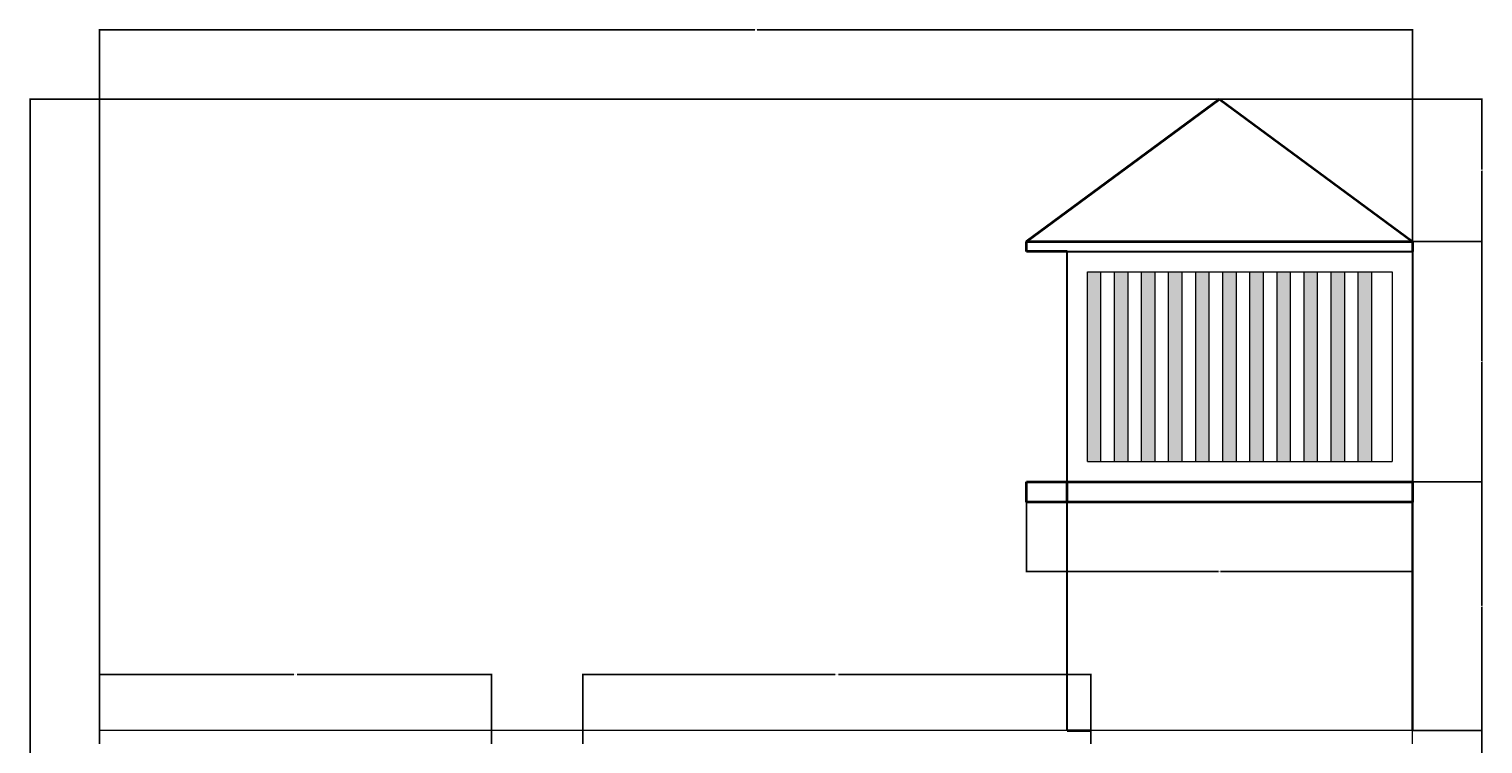
# Model space of a CAD drawing. Units: inches. Extents: x 2156 to 3149, y 1513 to 2286.
# Tile 5 of 5: x 2720 to 3149, y 2075 to 2286. Entities that reach past the tile are written whole.
import ezdxf

# ---------------------------------------------------------------- set-up
doc = ezdxf.new("R2010")
doc.units = ezdxf.units.IN
for name, color, linetype, lineweight in [('A-ANNO-DIMS', 2, 'Continuous', 18), ('A-ELEV', 7, 'Continuous', 30), ('A-ELEV-GLAZ', 4, 'Continuous', 18), ('A-ELEV-GLAZ-PATT', 18, 'Continuous', 13), ('A-ELEV-TRIM', 7, 'Continuous', 20), ('A-ROOF', 7, 'Continuous', 35)]:
    doc.layers.add(name, color=color, linetype=linetype, lineweight=lineweight)
doc.styles.get("Standard").update_dxf_attribs({"font": 'arial.ttf'})
doc.dimstyles.get("Standard").update_dxf_attribs({"dimtxt": 0.18, "dimasz": 0.18, "dimexe": 0.18, "dimexo": 0.0625, "dimgap": 0.09, "dimtad": 0, "dimtih": 1, "dimtoh": 1, "dimdec": 4, "dimzin": 0, "dimdsep": 46, "dimtxsty": 'Standard', "dimcen": 0.09, "dimadec": 0, "dimazin": 0, "dimtfac": 1, "dimtdec": 4, "dimtofl": 0, "dimtmove": 0, "dimatfit": 3, "dimfxl": 1, "dimtolj": 1, "dimtzin": 0, "dimarcsym": 0})

# ---------------------------------------------------------------- blocks, each defined once
blk = doc.blocks.new('*D45')
at = {"layer": 'A-ANNO-DIMS', "color": 0, "lineweight": -2, "transparency": 16777216}
for p, q in [((2740.82, 2078.77), (2740.82, 2285.77)), ((2741, 2285.59), (2934.28, 2285.59)), ((3128.35, 2285.59), (2935.06, 2285.59)), ((3128.53, 2223.16), (3128.53, 2285.77))]:
    blk.add_line(p, q, dxfattribs=at)
at = {"layer": 'A-ANNO-DIMS', "color": 0, "transparency": 16777216}
for points in [[(2741, 2285.62), (2741, 2285.56), (2740.82, 2285.59)], [(3128.35, 2285.62), (3128.35, 2285.56), (3128.53, 2285.59)]]:
    blk.add_solid(points, dxfattribs=at)
at = {"layer": 'Defpoints', "color": 0, "transparency": 16777216}
for p in [(3128.53, 2285.59), (3128.53, 2223.09), (2740.82, 2078.71)]:
    blk.add_point(p, dxfattribs=at)
at = {"layer": 'A-ANNO-DIMS', "color": 0, "transparency": 16777216, "insert": (2934.67, 2285.59), "char_height": 0.18, "attachment_point": 5}
blk.add_mtext('\\A1;387.7', dxfattribs=at)
blk = doc.blocks.new('*D46')
at = {"layer": 'A-ANNO-DIMS', "color": 0, "lineweight": -2, "transparency": 16777216}
for p, q in [((3071.46, 2265.09), (2720.14, 2265.09)), ((2720.32, 2264.91), (2720.32, 2062.08)), ((2720.32, 1858.89), (2720.32, 2061.72)), ((2740.75, 1858.71), (2720.14, 1858.71))]:
    blk.add_line(p, q, dxfattribs=at)
at = {"layer": 'A-ANNO-DIMS', "color": 0, "transparency": 16777216}
for points in [[(2720.29, 2264.91), (2720.35, 2264.91), (2720.32, 2265.09)], [(2720.29, 1858.89), (2720.35, 1858.89), (2720.32, 1858.71)]]:
    blk.add_solid(points, dxfattribs=at)
at = {"layer": 'Defpoints', "color": 0, "transparency": 16777216}
for p in [(2720.32, 2265.09), (3071.53, 2265.09), (2740.82, 1858.71)]:
    blk.add_point(p, dxfattribs=at)
at = {"layer": 'A-ANNO-DIMS', "color": 0, "transparency": 16777216, "insert": (2720.32, 2061.9), "char_height": 0.18, "attachment_point": 5}
blk.add_mtext('\\A1;406.4', dxfattribs=at)
blk = doc.blocks.new('*D47')
at = {"layer": 'A-ANNO-DIMS', "color": 0, "lineweight": -2, "transparency": 16777216}
for p, q in [((3014.53, 2146.03), (3014.53, 2125.41)), ((3128.53, 2146.03), (3128.53, 2125.41)), ((3014.71, 2125.59), (3071.25, 2125.59)), ((3128.35, 2125.59), (3071.81, 2125.59))]:
    blk.add_line(p, q, dxfattribs=at)
at = {"layer": 'A-ANNO-DIMS', "color": 0, "transparency": 16777216}
for points in [[(3014.71, 2125.62), (3014.71, 2125.56), (3014.53, 2125.59)], [(3128.35, 2125.62), (3128.35, 2125.56), (3128.53, 2125.59)]]:
    blk.add_solid(points, dxfattribs=at)
at = {"layer": 'Defpoints', "color": 0, "transparency": 16777216}
for p in [(3014.53, 2146.09), (3128.53, 2146.09), (3014.53, 2125.59)]:
    blk.add_point(p, dxfattribs=at)
at = {"layer": 'A-ANNO-DIMS', "color": 0, "transparency": 16777216, "insert": (3071.53, 2125.59), "char_height": 0.18, "attachment_point": 5}
blk.add_mtext('\\A1;114', dxfattribs=at)
blk = doc.blocks.new('*D49')
at = {"layer": 'A-ANNO-DIMS', "color": 0, "lineweight": -2, "transparency": 16777216}
for p, q in [((2740.82, 2074.77), (2740.82, 2095.39)), ((2741, 2095.21), (2798.23, 2095.21)), ((2856.37, 2095.21), (2799.14, 2095.21)), ((2856.55, 2074.77), (2856.55, 2095.39))]:
    blk.add_line(p, q, dxfattribs=at)
at = {"layer": 'A-ANNO-DIMS', "color": 0, "transparency": 16777216}
for points in [[(2741, 2095.24), (2741, 2095.18), (2740.82, 2095.21)], [(2856.37, 2095.24), (2856.37, 2095.18), (2856.55, 2095.21)]]:
    blk.add_solid(points, dxfattribs=at)
at = {"layer": 'Defpoints', "color": 0, "transparency": 16777216}
for p in [(2856.55, 2095.21), (2740.82, 2074.71), (2856.55, 2074.71)]:
    blk.add_point(p, dxfattribs=at)
at = {"layer": 'A-ANNO-DIMS', "color": 0, "transparency": 16777216, "insert": (2798.68, 2095.21), "char_height": 0.18, "attachment_point": 5}
blk.add_mtext('\\A1;115.74', dxfattribs=at)
blk = doc.blocks.new('*D50')
at = {"layer": 'A-ANNO-DIMS', "color": 0, "lineweight": -2, "transparency": 16777216}
for p, q in [((2883.55, 2074.77), (2883.55, 2095.39)), ((2883.73, 2095.21), (2958.08, 2095.21)), ((3033.35, 2095.21), (2958.99, 2095.21)), ((3033.53, 2074.77), (3033.53, 2095.39))]:
    blk.add_line(p, q, dxfattribs=at)
at = {"layer": 'A-ANNO-DIMS', "color": 0, "transparency": 16777216}
for points in [[(2883.73, 2095.24), (2883.73, 2095.18), (2883.55, 2095.21)], [(3033.35, 2095.24), (3033.35, 2095.18), (3033.53, 2095.21)]]:
    blk.add_solid(points, dxfattribs=at)
at = {"layer": 'Defpoints', "color": 0, "transparency": 16777216}
for p in [(3033.53, 2095.21), (2883.55, 2074.71), (3033.53, 2074.71)]:
    blk.add_point(p, dxfattribs=at)
at = {"layer": 'A-ANNO-DIMS', "color": 0, "transparency": 16777216, "insert": (2958.54, 2095.21), "char_height": 0.18, "attachment_point": 5}
blk.add_mtext('\\A1;149.97', dxfattribs=at)
blk = doc.blocks.new('*D54')
at = {"layer": 'A-ANNO-DIMS', "color": 0, "lineweight": -2, "transparency": 16777216}
for p, q in [((3128.59, 2078.71), (3149.21, 2078.71)), ((3149.03, 2078.53), (3149.03, 2028.89)), ((3149.03, 1978.89), (3149.03, 2028.53)), ((2998.09, 1978.71), (3149.21, 1978.71))]:
    blk.add_line(p, q, dxfattribs=at)
at = {"layer": 'A-ANNO-DIMS', "color": 0, "transparency": 16777216}
for points in [[(3149, 2078.53), (3149.06, 2078.53), (3149.03, 2078.71)], [(3149, 1978.89), (3149.06, 1978.89), (3149.03, 1978.71)]]:
    blk.add_solid(points, dxfattribs=at)
at = {"layer": 'Defpoints', "color": 0, "transparency": 16777216}
for p in [(3128.53, 2078.71), (3149.03, 2078.71), (2998.03, 1978.71)]:
    blk.add_point(p, dxfattribs=at)
at = {"layer": 'A-ANNO-DIMS', "color": 0, "transparency": 16777216, "insert": (3149.03, 2028.71), "char_height": 0.18, "attachment_point": 5}
blk.add_mtext('\\A1;100', dxfattribs=at)
blk = doc.blocks.new('*D55')
at = {"layer": 'A-ANNO-DIMS', "color": 0, "lineweight": -2, "transparency": 16777216}
for p, q in [((3128.59, 2152.09), (3149.21, 2152.09)), ((3149.03, 2151.91), (3149.03, 2115.58)), ((3149.03, 2078.89), (3149.03, 2115.22)), ((3128.59, 2078.71), (3149.21, 2078.71))]:
    blk.add_line(p, q, dxfattribs=at)
at = {"layer": 'A-ANNO-DIMS', "color": 0, "transparency": 16777216}
for points in [[(3149, 2151.91), (3149.06, 2151.91), (3149.03, 2152.09)], [(3149, 2078.89), (3149.06, 2078.89), (3149.03, 2078.71)]]:
    blk.add_solid(points, dxfattribs=at)
at = {"layer": 'Defpoints', "color": 0, "transparency": 16777216}
for p in [(3128.53, 2152.09), (3149.03, 2152.09), (3128.53, 2078.71)]:
    blk.add_point(p, dxfattribs=at)
at = {"layer": 'A-ANNO-DIMS', "color": 0, "transparency": 16777216, "insert": (3149.03, 2115.4), "char_height": 0.18, "attachment_point": 5}
blk.add_mtext('\\A1;73.39', dxfattribs=at)
blk = doc.blocks.new('*D56')
at = {"layer": 'A-ANNO-DIMS', "color": 0, "lineweight": -2, "transparency": 16777216}
for p, q in [((3128.59, 2223.09), (3149.21, 2223.09)), ((3149.03, 2222.91), (3149.03, 2187.77)), ((3149.03, 2152.27), (3149.03, 2187.41)), ((3128.59, 2152.09), (3149.21, 2152.09))]:
    blk.add_line(p, q, dxfattribs=at)
at = {"layer": 'A-ANNO-DIMS', "color": 0, "transparency": 16777216}
for points in [[(3149, 2222.91), (3149.06, 2222.91), (3149.03, 2223.09)], [(3149, 2152.27), (3149.06, 2152.27), (3149.03, 2152.09)]]:
    blk.add_solid(points, dxfattribs=at)
at = {"layer": 'Defpoints', "color": 0, "transparency": 16777216}
for p in [(3128.53, 2223.09), (3149.03, 2223.09), (3128.53, 2152.09)]:
    blk.add_point(p, dxfattribs=at)
at = {"layer": 'A-ANNO-DIMS', "color": 0, "transparency": 16777216, "insert": (3149.03, 2187.59), "char_height": 0.18, "attachment_point": 5}
blk.add_mtext('\\A1;71', dxfattribs=at)
blk = doc.blocks.new('*D57')
at = {"layer": 'A-ANNO-DIMS', "color": 0, "lineweight": -2, "transparency": 16777216}
for p, q in [((3071.59, 2265.09), (3149.21, 2265.09)), ((3149.03, 2264.91), (3149.03, 2244.27)), ((3149.03, 2223.27), (3149.03, 2243.91)), ((3128.59, 2223.09), (3149.21, 2223.09))]:
    blk.add_line(p, q, dxfattribs=at)
at = {"layer": 'A-ANNO-DIMS', "color": 0, "transparency": 16777216}
for points in [[(3149, 2264.91), (3149.06, 2264.91), (3149.03, 2265.09)], [(3149, 2223.27), (3149.06, 2223.27), (3149.03, 2223.09)]]:
    blk.add_solid(points, dxfattribs=at)
at = {"layer": 'Defpoints', "color": 0, "transparency": 16777216}
for p in [(3071.53, 2265.09), (3149.03, 2265.09), (3128.53, 2223.09)]:
    blk.add_point(p, dxfattribs=at)
at = {"layer": 'A-ANNO-DIMS', "color": 0, "transparency": 16777216, "insert": (3149.03, 2244.09), "char_height": 0.18, "attachment_point": 5}
blk.add_mtext('\\A1;42', dxfattribs=at)

msp = doc.modelspace()

# ---------------------------------------------------------------- hatches: boundary and pattern name
at = {"layer": 'A-ELEV-GLAZ-PATT'}
h = msp.add_hatch(color=256, dxfattribs=at)
h.dxf.hatch_style = 1
h.paths.add_polyline_path([(3036.526, 2214.094), (3032.526, 2214.094), (3032.526, 2158.094), (3036.526, 2158.094)])
h.paths.add_polyline_path([(3044.526, 2214.094), (3040.526, 2214.094), (3040.526, 2158.094), (3044.526, 2158.094)])
h.paths.add_polyline_path([(3052.526, 2214.094), (3048.526, 2214.094), (3048.526, 2158.094), (3052.526, 2158.094)])
h.paths.add_polyline_path([(3060.526, 2214.094), (3056.526, 2214.094), (3056.526, 2158.094), (3060.526, 2158.094)])
h.paths.add_polyline_path([(3068.526, 2214.094), (3064.526, 2214.094), (3064.526, 2158.094), (3068.526, 2158.094)])
h.paths.add_polyline_path([(3076.526, 2214.094), (3072.526, 2214.094), (3072.526, 2158.094), (3076.526, 2158.094)])
h.paths.add_polyline_path([(3084.526, 2214.094), (3080.526, 2214.094), (3080.526, 2158.094), (3084.526, 2158.094)])
h.paths.add_polyline_path([(3092.526, 2214.094), (3088.526, 2214.094), (3088.526, 2158.094), (3092.526, 2158.094)])
h.paths.add_polyline_path([(3100.526, 2214.094), (3096.526, 2214.094), (3096.526, 2158.094), (3100.526, 2158.094)])
h.paths.add_polyline_path([(3108.526, 2214.094), (3104.526, 2214.094), (3104.526, 2158.094), (3108.526, 2158.094)])
h.paths.add_polyline_path([(3116.526, 2214.094), (3112.526, 2214.094), (3112.526, 2158.094), (3116.526, 2158.094)])

# ---------------------------------------------------------------- linework, layer by layer
at = {"layer": 'A-ELEV'}
for p, q in [((3026.526, 2152.094), (3026.526, 2220.094)), ((3026.526, 2220.094), (3128.526, 2220.094)), ((3128.526, 2220.094), (3128.526, 2152.094)), ((3128.526, 2152.094), (3128.526, 2078.708)), ((3128.526, 2078.708), (3128.526, 2152.094)), ((3026.526, 2128.094), (3026.526, 2146.094)), ((3026.526, 2078.708), (3026.526, 2128.094))]:
    msp.add_line(p, q, dxfattribs=at)
at = {"layer": 'A-ELEV-GLAZ'}
for p, q in [((3032.526, 2158.094), (3032.526, 2214.094)), ((3032.526, 2214.094), (3122.526, 2214.094)), ((3036.526, 2158.094), (3036.526, 2214.094)), ((3040.526, 2158.094), (3040.526, 2214.094)), ((3044.526, 2158.094), (3044.526, 2214.094)), ((3048.526, 2158.094), (3048.526, 2214.094)), ((3052.526, 2158.094), (3052.526, 2214.094)), ((3056.526, 2158.094), (3056.526, 2214.094)), ((3060.526, 2158.094), (3060.526, 2214.094)), ((3064.526, 2158.094), (3064.526, 2214.094)), ((3068.526, 2158.094), (3068.526, 2214.094)), ((3072.526, 2158.094), (3072.526, 2214.094)), ((3076.526, 2158.094), (3076.526, 2214.094)), ((3080.526, 2158.094), (3080.526, 2214.094)), ((3084.526, 2158.094), (3084.526, 2214.094)), ((3088.526, 2158.094), (3088.526, 2214.094)), ((3092.526, 2158.094), (3092.526, 2214.094)), ((3096.526, 2158.094), (3096.526, 2214.094)), ((3100.526, 2158.094), (3100.526, 2214.094)), ((3104.526, 2158.094), (3104.526, 2214.094)), ((3108.526, 2158.094), (3108.526, 2214.094)), ((3112.526, 2158.094), (3112.526, 2214.094)), ((3116.526, 2158.094), (3116.526, 2214.094)), ((3122.526, 2214.094), (3122.526, 2158.094)), ((3032.526, 2158.094), (3122.526, 2158.094))]:
    msp.add_line(p, q, dxfattribs=at)
at = {"layer": 'A-ELEV-TRIM'}
for p, q in [((2828.526, 2078.708), (2740.816, 2078.708)), ((2740.816, 2078.708), (2740.816, 2074.708)), ((3128.526, 2078.708), (2828.526, 2078.708)), ((3128.526, 2074.708), (3128.526, 2078.708))]:
    msp.add_line(p, q, dxfattribs=at)
at = {"layer": 'A-ROOF'}
for p, q in [((3071.526, 2265.094), (3014.526, 2223.094)), ((3014.526, 2223.094), (3071.526, 2265.094)), ((3071.526, 2265.094), (3128.526, 2223.094)), ((3014.526, 2220.094), (3014.526, 2223.094)), ((3014.526, 2223.094), (3128.526, 2223.094)), ((3026.526, 2220.094), (3014.526, 2220.094)), ((3128.526, 2223.094), (3128.526, 2220.094)), ((3014.526, 2146.094), (3014.526, 2152.094)), ((3014.526, 2152.094), (3128.526, 2152.094)), ((3026.526, 2146.094), (3026.526, 2152.094)), ((3128.526, 2152.094), (3128.526, 2146.094)), ((3026.526, 2146.094), (3014.526, 2146.094)), ((3128.526, 2146.094), (3026.526, 2146.094)), ((3026.526, 2078.708), (3033.526, 2078.708))]:
    msp.add_line(p, q, dxfattribs=at)

# ---------------------------------------------------------------- dimensions: what is measured, and where the dimension line sits
at = {"layer": 'A-ANNO-DIMS'}
for base, p1, p2, override, picture, middle in [((3128.526, 2285.594), (2740.816, 2078.708), (3128.526, 2223.094), {"dimdec": 1, "dimlfac": 1, "dimrnd": 0, "dimzin": 0, "dimdsep": 46, "dimlunit": 2}, '*D45', (2934.671, 2285.594)), ((2856.553, 2095.208), (2740.816, 2074.708), (2856.553, 2074.708), {"dimdec": 2, "dimlfac": 1, "dimrnd": 0, "dimzin": 0, "dimdsep": 46, "dimlunit": 2}, '*D49', (2798.684, 2095.208)), ((3033.526, 2095.208), (2883.553, 2074.708), (3033.526, 2074.708), {"dimdec": 2, "dimlfac": 1, "dimrnd": 0, "dimzin": 0, "dimdsep": 46, "dimlunit": 2}, '*D50', (2958.539, 2095.208))]:
    dim = msp.add_linear_dim(base=base, p1=p1, p2=p2, dimstyle='Standard', override=override, dxfattribs=at)
    dim.commit()
    dim.dimension.update_dxf_attribs({"geometry": picture, "text_midpoint": middle})
for base, p1, p2, angle, override, picture, middle in [((2720.316, 2265.094), (2740.816, 1858.708), (3071.526, 2265.094), 90, {"dimdec": 1, "dimlfac": 1, "dimrnd": 0, "dimzin": 0, "dimdsep": 46, "dimlunit": 2}, '*D46', (2720.316, 2061.901)), ((3149.026, 2265.094), (3128.526, 2223.094), (3071.526, 2265.094), 90, {"dimdec": 0, "dimlfac": 1, "dimrnd": 0, "dimzin": 0, "dimdsep": 46, "dimlunit": 2}, '*D57', (3149.026, 2244.094)), ((3149.026, 2223.094), (3128.526, 2152.094), (3128.526, 2223.094), 90, {"dimdec": 0, "dimlfac": 1, "dimrnd": 0, "dimzin": 0, "dimdsep": 46, "dimlunit": 2}, '*D56', (3149.026, 2187.594)), ((3149.026, 2152.094), (3128.526, 2078.708), (3128.526, 2152.094), 90, {"dimdec": 2, "dimlfac": 1, "dimrnd": 0, "dimzin": 0, "dimdsep": 46, "dimlunit": 2}, '*D55', (3149.026, 2115.401)), ((3014.526, 2125.594), (3128.526, 2146.094), (3014.526, 2146.094), 180, {"dimdec": 0, "dimlfac": 1, "dimrnd": 0, "dimzin": 0, "dimdsep": 46, "dimlunit": 2}, '*D47', (3071.526, 2125.594)), ((3149.026, 2078.708), (2998.026, 1978.708), (3128.526, 2078.708), 90, {"dimdec": 0, "dimlfac": 1, "dimrnd": 0, "dimzin": 0, "dimdsep": 46, "dimlunit": 2}, '*D54', (3149.026, 2028.708))]:
    dim = msp.add_linear_dim(base=base, p1=p1, p2=p2, angle=angle, dimstyle='Standard', override=override, dxfattribs=at)
    dim.commit()
    dim.dimension.update_dxf_attribs({"geometry": picture, "text_midpoint": middle})

doc.saveas('drawing.dxf')
